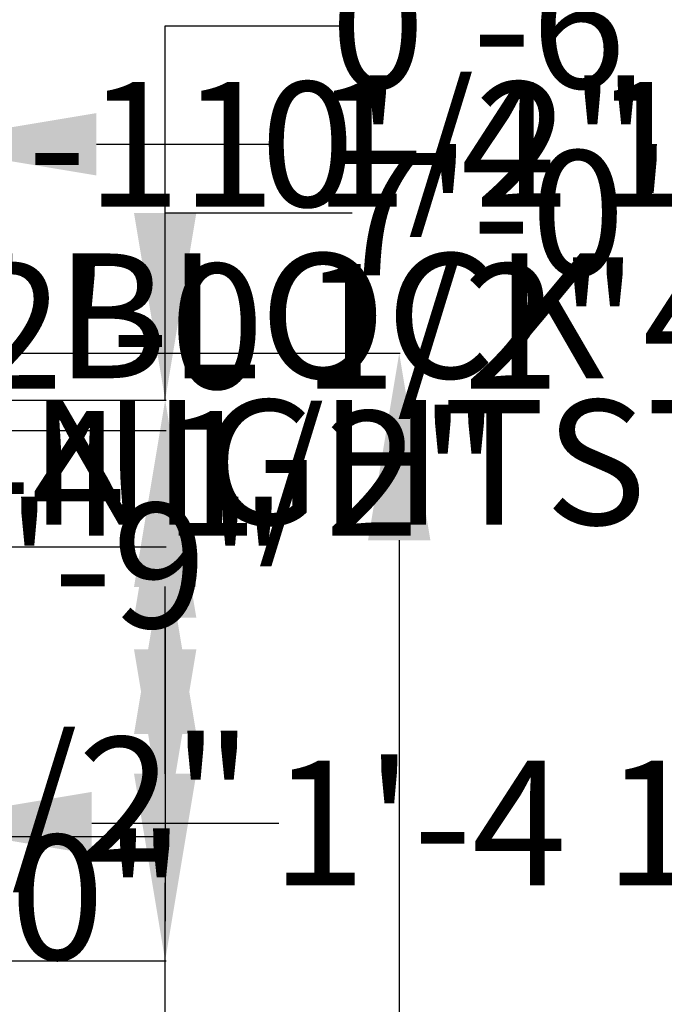
# Model space of a CAD drawing. Units: inches. Extents: x 2838 to 4029, y 1041 to 1915.
# Tile 14 of 16: x 3640 to 3764, y 1546 to 1735. Entities that reach past the tile are written whole.
import ezdxf

# ---------------------------------------------------------------- set-up
doc = ezdxf.new("R2010")
doc.units = ezdxf.units.IN
doc.header["$MEASUREMENT"] = 0
doc.layers.add('A-ANNO-DIMS', color=2, linetype='Continuous', lineweight=18)
doc.styles.get("Standard").update_dxf_attribs({"font": 'arial.ttf'})
doc.dimstyles.get("Standard").update_dxf_attribs({"dimtxt": 24, "dimasz": 36, "dimexe": 0.18, "dimexo": 0.0625, "dimgap": 0.09, "dimtad": 0, "dimtih": 1, "dimtoh": 1, "dimdec": 0, "dimzin": 0, "dimdsep": 46, "dimlunit": 3, "dimtxsty": 'Standard', "dimcen": 0.09, "dimadec": 0, "dimazin": 0, "dimtfac": 1, "dimtdec": 0, "dimtofl": 0, "dimtmove": 0, "dimatfit": 3, "dimfxl": 1, "dimtolj": 1, "dimtzin": 0, "dimarcsym": 0})

# ---------------------------------------------------------------- blocks, each defined once
blk = doc.blocks.new('*D17')
at = {"layer": 'A-ANNO-DIMS', "color": 0, "lineweight": -2, "transparency": 16777216}
for p, q in [((3627.79, 1671.3), (3713.18, 1671.3)), ((3713, 1635.3), (3713, 1443.64)), ((3713, 1227.3), (3713, 1418.95)), ((3627.79, 1191.3), (3713.18, 1191.3))]:
    blk.add_line(p, q, dxfattribs=at)
at = {"layer": 'A-ANNO-DIMS', "color": 0, "transparency": 16777216}
for points in [[(3707, 1635.3), (3719, 1635.3), (3713, 1671.3)], [(3707, 1227.3), (3719, 1227.3), (3713, 1191.3)]]:
    blk.add_solid(points, dxfattribs=at)
at = {"layer": 'Defpoints', "color": 0, "transparency": 16777216}
for p in [(3627.73, 1671.3), (3627.73, 1191.3), (3713, 1191.3)]:
    blk.add_point(p, dxfattribs=at)
at = {"layer": 'A-ANNO-DIMS', "color": 0, "transparency": 16777216, "insert": (3713, 1431.3), "char_height": 24, "attachment_point": 5}
blk.add_mtext("\\A1;40'", dxfattribs=at)
blk = doc.blocks.new('*D27')
at = {"layer": 'A-ANNO-DIMS', "color": 0, "lineweight": -2, "transparency": 16777216}
for p, q in [((3598.68, 1614.31), (3598.68, 1650.31)), ((3598.68, 1650.31), (3634.68, 1650.31)), ((3601.19, 1578.31), (3598.5, 1578.31)), ((3601.19, 1561.16), (3598.5, 1561.16)), ((3598.68, 1525.16), (3598.68, 1489.16))]:
    blk.add_line(p, q, dxfattribs=at)
at = {"layer": 'A-ANNO-DIMS', "color": 0, "transparency": 16777216}
for points in [[(3592.68, 1614.31), (3604.68, 1614.31), (3598.68, 1578.31)], [(3592.68, 1525.16), (3604.68, 1525.16), (3598.68, 1561.16)]]:
    blk.add_solid(points, dxfattribs=at)
at = {"layer": 'Defpoints', "color": 0, "transparency": 16777216}
for p in [(3598.68, 1578.31), (3601.25, 1578.31), (3601.25, 1561.16)]:
    blk.add_point(p, dxfattribs=at)
at = {"layer": 'A-ANNO-DIMS', "color": 0, "transparency": 16777216, "insert": (3820.96, 1650.31), "char_height": 24, "attachment_point": 5}
blk.add_mtext('\\A1;NIGHTSTAND 1\'-5" TYP.', dxfattribs=at)
blk = doc.blocks.new('*D28')
at = {"layer": 'A-ANNO-DIMS', "color": 0, "lineweight": -2, "transparency": 16777216}
for p, q in [((3565.25, 1580.88), (3529.25, 1580.88)), ((3601.25, 1578.37), (3601.25, 1581.06)), ((3617.82, 1578.37), (3617.82, 1581.06)), ((3653.82, 1580.88), (3689.82, 1580.88))]:
    blk.add_line(p, q, dxfattribs=at)
at = {"layer": 'A-ANNO-DIMS', "color": 0, "transparency": 16777216}
for points in [[(3565.25, 1586.88), (3565.25, 1574.88), (3601.25, 1580.88)], [(3653.82, 1586.88), (3653.82, 1574.88), (3617.82, 1580.88)]]:
    blk.add_solid(points, dxfattribs=at)
at = {"layer": 'Defpoints', "color": 0, "transparency": 16777216}
for p in [(3617.82, 1580.88), (3601.25, 1578.31), (3617.82, 1578.31)]:
    blk.add_point(p, dxfattribs=at)
at = {"layer": 'A-ANNO-DIMS', "color": 0, "transparency": 16777216, "insert": (3789.89, 1580.88), "char_height": 24, "attachment_point": 5}
blk.add_mtext('\\A1;1\'-4 1/2" TYP.', dxfattribs=at)
blk = doc.blocks.new('*D36')
at = {"layer": 'A-ANNO-DIMS', "color": 0, "lineweight": -2, "transparency": 16777216}
for p, q in [((3481.95, 1586.87), (3481.95, 1585.25)), ((3488.45, 1586.87), (3488.45, 1585.25)), ((3445.95, 1585.43), (3409.95, 1585.43)), ((3524.45, 1585.43), (3560.45, 1585.43))]:
    blk.add_line(p, q, dxfattribs=at)
at = {"layer": 'A-ANNO-DIMS', "color": 0, "transparency": 16777216}
for points in [[(3445.95, 1591.43), (3445.95, 1579.43), (3481.95, 1585.43)], [(3524.45, 1591.43), (3524.45, 1579.43), (3488.45, 1585.43)]]:
    blk.add_solid(points, dxfattribs=at)
at = {"layer": 'Defpoints', "color": 0, "transparency": 16777216}
for p in [(3481.95, 1586.93), (3488.45, 1586.93), (3488.45, 1585.43)]:
    blk.add_point(p, dxfattribs=at)
at = {"layer": 'A-ANNO-DIMS', "color": 0, "transparency": 16777216, "insert": (3620.4, 1585.43), "char_height": 24, "attachment_point": 5}
blk.add_mtext('\\A1;0\'-6 1/2"', dxfattribs=at)
blk = doc.blocks.new('*D39')
at = {"layer": 'A-ANNO-DIMS', "color": 0, "lineweight": -2, "transparency": 16777216}
for p, q in [((3391.52, 1678.5), (3355.52, 1678.5)), ((3427.52, 1671.36), (3427.52, 1678.68)), ((3475.52, 1671.36), (3475.52, 1678.68)), ((3511.52, 1678.5), (3547.52, 1678.5))]:
    blk.add_line(p, q, dxfattribs=at)
at = {"layer": 'A-ANNO-DIMS', "color": 0, "transparency": 16777216}
for points in [[(3391.52, 1684.5), (3391.52, 1672.5), (3427.52, 1678.5)], [(3511.52, 1684.5), (3511.52, 1672.5), (3475.52, 1678.5)]]:
    blk.add_solid(points, dxfattribs=at)
at = {"layer": 'Defpoints', "color": 0, "transparency": 16777216}
for p in [(3475.52, 1678.5), (3427.52, 1671.3), (3475.52, 1671.3)]:
    blk.add_point(p, dxfattribs=at)
at = {"layer": 'A-ANNO-DIMS', "color": 0, "transparency": 16777216, "insert": (3732.24, 1678.5), "char_height": 24, "attachment_point": 5}
blk.add_mtext('\\A1;VENT BLOCK 4\'-0" TYP.', dxfattribs=at)
blk = doc.blocks.new('*D41')
at = {"layer": 'A-ANNO-DIMS', "color": 0, "lineweight": -2, "transparency": 16777216}
for p, q in [((3284.24, 1506.2), (3284.24, 1496.56)), ((3347.73, 1506.2), (3347.73, 1496.56)), ((3248.24, 1496.74), (3212.24, 1496.74)), ((3383.73, 1496.74), (3419.73, 1496.74))]:
    blk.add_line(p, q, dxfattribs=at)
at = {"layer": 'A-ANNO-DIMS', "color": 0, "transparency": 16777216}
for points in [[(3248.24, 1502.74), (3248.24, 1490.74), (3284.24, 1496.74)], [(3383.73, 1502.74), (3383.73, 1490.74), (3347.73, 1496.74)]]:
    blk.add_solid(points, dxfattribs=at)
at = {"layer": 'Defpoints', "color": 0, "transparency": 16777216}
for p in [(3284.24, 1506.26), (3347.73, 1506.26), (3347.73, 1496.74)]:
    blk.add_point(p, dxfattribs=at)
at = {"layer": 'A-ANNO-DIMS', "color": 0, "transparency": 16777216, "insert": (3624.81, 1496.74), "char_height": 24, "attachment_point": 5}
blk.add_mtext('\\A1;WARDROBE 5\'-3 1/2" TYP.', dxfattribs=at)
blk = doc.blocks.new('*D45')
at = {"layer": 'A-ANNO-DIMS', "color": 0, "lineweight": -2, "transparency": 16777216}
for p, q in [((3456.69, 1635.35), (3456.69, 1630.27)), ((3489.73, 1635.35), (3489.73, 1630.27)), ((3420.69, 1630.45), (3384.69, 1630.45)), ((3525.73, 1630.45), (3561.73, 1630.45))]:
    blk.add_line(p, q, dxfattribs=at)
at = {"layer": 'A-ANNO-DIMS', "color": 0, "transparency": 16777216}
for points in [[(3420.69, 1636.45), (3420.69, 1624.45), (3456.69, 1630.45)], [(3525.73, 1636.45), (3525.73, 1624.45), (3489.73, 1630.45)]]:
    blk.add_solid(points, dxfattribs=at)
at = {"layer": 'Defpoints', "color": 0, "transparency": 16777216}
for p in [(3456.69, 1635.41), (3489.73, 1635.41), (3489.73, 1630.45)]:
    blk.add_point(p, dxfattribs=at)
at = {"layer": 'A-ANNO-DIMS', "color": 0, "transparency": 16777216, "insert": (3626.8, 1630.45), "char_height": 24, "attachment_point": 5}
blk.add_mtext('\\A1;WC 2\'-9"', dxfattribs=at)
blk = doc.blocks.new('*D47')
at = {"layer": 'A-ANNO-DIMS', "color": 0, "lineweight": -2, "transparency": 16777216}
for p, q in [((3493.47, 1640.5), (3493.47, 1676.5)), ((3493.47, 1676.5), (3529.47, 1676.5)), ((3489.85, 1604.5), (3493.65, 1604.5)), ((3489.85, 1579.95), (3493.65, 1579.95)), ((3493.47, 1543.95), (3493.47, 1507.95))]:
    blk.add_line(p, q, dxfattribs=at)
at = {"layer": 'A-ANNO-DIMS', "color": 0, "transparency": 16777216}
for points in [[(3487.47, 1640.5), (3499.47, 1640.5), (3493.47, 1604.5)], [(3487.47, 1543.95), (3499.47, 1543.95), (3493.47, 1579.95)]]:
    blk.add_solid(points, dxfattribs=at)
at = {"layer": 'Defpoints', "color": 0, "transparency": 16777216}
for p in [(3489.78, 1604.5), (3493.47, 1604.5), (3489.78, 1579.95)]:
    blk.add_point(p, dxfattribs=at)
at = {"layer": 'A-ANNO-DIMS', "color": 0, "transparency": 16777216, "insert": (3643.85, 1676.5), "char_height": 24, "attachment_point": 5}
blk.add_mtext('\\A1;BASIN 2\'-0 1/2"', dxfattribs=at)
blk = doc.blocks.new('*D56')
at = {"layer": 'A-ANNO-DIMS', "color": 0, "lineweight": -2, "transparency": 16777216}
for p, q in [((3567.44, 1530.6), (3567.44, 1566.6)), ((3567.44, 1566.6), (3603.44, 1566.6)), ((3562.33, 1494.6), (3567.62, 1494.6)), ((3562.33, 1470.6), (3567.62, 1470.6)), ((3567.44, 1434.6), (3567.44, 1398.6))]:
    blk.add_line(p, q, dxfattribs=at)
at = {"layer": 'A-ANNO-DIMS', "color": 0, "transparency": 16777216}
for points in [[(3561.44, 1530.6), (3573.44, 1530.6), (3567.44, 1494.6)], [(3561.44, 1434.6), (3573.44, 1434.6), (3567.44, 1470.6)]]:
    blk.add_solid(points, dxfattribs=at)
at = {"layer": 'Defpoints', "color": 0, "transparency": 16777216}
for p in [(3562.26, 1494.6), (3567.44, 1494.6), (3562.26, 1470.6)]:
    blk.add_point(p, dxfattribs=at)
at = {"layer": 'A-ANNO-DIMS', "color": 0, "transparency": 16777216, "insert": (3635.63, 1566.6), "char_height": 24, "attachment_point": 5}
blk.add_mtext('\\A1;2\'-0"', dxfattribs=at)
blk = doc.blocks.new('*D73')
at = {"layer": 'A-ANNO-DIMS', "color": 0, "lineweight": -2, "transparency": 16777216}
for p, q in [((3425.038746, 1711.522346), (3389.038746, 1711.522346)), ((3461.038746, 1200.359846), (3461.038746, 1711.702346)), ((3618.731626, 1200.359846), (3618.731626, 1711.702346)), ((3654.731626, 1711.522346), (3690.731626, 1711.522346))]:
    blk.add_line(p, q, dxfattribs=at)
at = {"layer": 'A-ANNO-DIMS', "color": 0, "transparency": 16777216}
for points in [[(3425.038746, 1717.522346), (3425.038746, 1705.522346), (3461.038746, 1711.522346)], [(3654.731626, 1717.522346), (3654.731626, 1705.522346), (3618.731626, 1711.522346)]]:
    blk.add_solid(points, dxfattribs=at)
at = {"layer": 'Defpoints', "color": 0, "transparency": 16777216}
for p in [(3618.731626, 1711.522346), (3461.038746, 1200.297346), (3618.731626, 1200.297346)]:
    blk.add_point(p, dxfattribs=at)
at = {"layer": 'A-ANNO-DIMS', "color": 0, "transparency": 16777216, "insert": (3539.885186, 1711.522346), "char_height": 24, "attachment_point": 5}
blk.add_mtext('\\A1;13\'-1 1/2"', dxfattribs=at)
blk = doc.blocks.new('*D78')
at = {"layer": 'A-ANNO-DIMS', "color": 0, "lineweight": -2, "transparency": 16777216}
for p, q in [((3667.956626, 1590.394218), (3667.956626, 1626.394218)), ((3498.794126, 1554.394218), (3668.136626, 1554.394218)), ((3498.638013, 1506.394218), (3668.136626, 1506.394218)), ((3667.956626, 1470.394218), (3667.956626, 1434.394218))]:
    blk.add_line(p, q, dxfattribs=at)
at = {"layer": 'A-ANNO-DIMS', "color": 0, "transparency": 16777216}
for points in [[(3661.956626, 1590.394218), (3673.956626, 1590.394218), (3667.956626, 1554.394218)], [(3661.956626, 1470.394218), (3673.956626, 1470.394218), (3667.956626, 1506.394218)]]:
    blk.add_solid(points, dxfattribs=at)
at = {"layer": 'Defpoints', "color": 0, "transparency": 16777216}
for p in [(3498.731626, 1554.394218), (3667.956626, 1554.394218), (3498.575513, 1506.394218)]:
    blk.add_point(p, dxfattribs=at)
at = {"layer": 'A-ANNO-DIMS', "color": 0, "transparency": 16777216, "insert": (3667.956626, 1530.394218), "char_height": 24, "attachment_point": 5}
blk.add_mtext('\\A1;4\'-0"', dxfattribs=at)
blk = doc.blocks.new('*D84')
at = {"layer": 'A-ANNO-DIMS', "color": 0, "lineweight": -2, "transparency": 16777216}
for p, q in [((3667.96, 1662.3), (3667.96, 1698.3)), ((3667.96, 1698.3), (3703.96, 1698.3)), ((3489.79, 1662.3), (3668.14, 1662.3)), ((3667.96, 1614.3), (3667.96, 1626.3)), ((3489.79, 1578.3), (3668.14, 1578.3))]:
    blk.add_line(p, q, dxfattribs=at)
at = {"layer": 'A-ANNO-DIMS', "color": 0, "transparency": 16777216}
for points in [[(3661.96, 1626.3), (3673.96, 1626.3), (3667.96, 1662.3)], [(3661.96, 1614.3), (3673.96, 1614.3), (3667.96, 1578.3)]]:
    blk.add_solid(points, dxfattribs=at)
at = {"layer": 'Defpoints', "color": 0, "transparency": 16777216}
for p in [(3489.73, 1662.3), (3667.96, 1662.3), (3489.73, 1578.3)]:
    blk.add_point(p, dxfattribs=at)
at = {"layer": 'A-ANNO-DIMS', "color": 0, "transparency": 16777216, "insert": (3735.85, 1698.3), "char_height": 24, "attachment_point": 5}
blk.add_mtext('\\A1;7\'-0"', dxfattribs=at)
blk = doc.blocks.new('*D94')
at = {"layer": 'A-ANNO-DIMS', "color": 0, "lineweight": -2, "transparency": 16777216}
for p, q in [((3667.96, 1533.39), (3667.96, 1569.39)), ((3585.44, 1497.39), (3668.14, 1497.39)), ((3585.44, 1469.25), (3668.14, 1469.25)), ((3667.96, 1433.25), (3667.96, 1397.25))]:
    blk.add_line(p, q, dxfattribs=at)
at = {"layer": 'A-ANNO-DIMS', "color": 0, "transparency": 16777216}
for points in [[(3661.96, 1533.39), (3673.96, 1533.39), (3667.96, 1497.39)], [(3661.96, 1433.25), (3673.96, 1433.25), (3667.96, 1469.25)]]:
    blk.add_solid(points, dxfattribs=at)
at = {"layer": 'Defpoints', "color": 0, "transparency": 16777216}
for p in [(3585.37, 1497.39), (3585.37, 1469.25), (3667.96, 1469.25)]:
    blk.add_point(p, dxfattribs=at)
at = {"layer": 'A-ANNO-DIMS', "color": 0, "transparency": 16777216, "insert": (3667.96, 1483.32), "char_height": 24, "attachment_point": 5}
blk.add_mtext('\\A1;2\'-4"', dxfattribs=at)
blk = doc.blocks.new('*D96')
at = {"layer": 'A-ANNO-DIMS', "color": 0, "lineweight": -2, "transparency": 16777216}
for p, q in [((3462.73, 1711.52), (3426.73, 1711.52)), ((3498.73, 1662.36), (3498.73, 1711.7)), ((3546.42, 1662.36), (3546.42, 1711.7)), ((3582.42, 1711.52), (3618.42, 1711.52))]:
    blk.add_line(p, q, dxfattribs=at)
at = {"layer": 'A-ANNO-DIMS', "color": 0, "transparency": 16777216}
for points in [[(3462.73, 1717.52), (3462.73, 1705.52), (3498.73, 1711.52)], [(3582.42, 1717.52), (3582.42, 1705.52), (3546.42, 1711.52)]]:
    blk.add_solid(points, dxfattribs=at)
at = {"layer": 'Defpoints', "color": 0, "transparency": 16777216}
for p in [(3546.42, 1711.52), (3498.73, 1662.3), (3546.42, 1662.3)]:
    blk.add_point(p, dxfattribs=at)
at = {"layer": 'A-ANNO-DIMS', "color": 0, "transparency": 16777216, "insert": (3687.68, 1711.52), "char_height": 24, "attachment_point": 5}
blk.add_mtext('\\A1;3\'-11 1/2"', dxfattribs=at)
blk = doc.blocks.new('*D97')
at = {"layer": 'A-ANNO-DIMS', "color": 0, "lineweight": -2, "transparency": 16777216}
for p, q in [((3667.956626, 1698.297346), (3667.956626, 1734.297346)), ((3618.794126, 1662.297346), (3668.136626, 1662.297346)), ((3618.794126, 1634.032994), (3668.136626, 1634.032994)), ((3667.956626, 1598.032994), (3667.956626, 1562.032994))]:
    blk.add_line(p, q, dxfattribs=at)
at = {"layer": 'A-ANNO-DIMS', "color": 0, "transparency": 16777216}
for points in [[(3661.956626, 1698.297346), (3673.956626, 1698.297346), (3667.956626, 1662.297346)], [(3661.956626, 1598.032994), (3673.956626, 1598.032994), (3667.956626, 1634.032994)]]:
    blk.add_solid(points, dxfattribs=at)
at = {"layer": 'Defpoints', "color": 0, "transparency": 16777216}
for p in [(3618.731626, 1662.297346), (3618.731626, 1634.032994), (3667.956626, 1634.032994)]:
    blk.add_point(p, dxfattribs=at)
at = {"layer": 'A-ANNO-DIMS', "color": 0, "transparency": 16777216, "insert": (3667.956626, 1648.16517), "char_height": 24, "attachment_point": 5}
blk.add_mtext('\\A1;2\'-4 1/2"', dxfattribs=at)
blk = doc.blocks.new('*D102')
at = {"layer": 'A-ANNO-DIMS', "color": 0, "lineweight": -2, "transparency": 16777216}
for p, q in [((3667.96, 1698.3), (3667.96, 1734.3)), ((3667.96, 1734.3), (3703.96, 1734.3)), ((3489.79, 1662.3), (3668.14, 1662.3)), ((3489.79, 1656.41), (3668.14, 1656.41)), ((3667.96, 1620.41), (3667.96, 1584.41))]:
    blk.add_line(p, q, dxfattribs=at)
at = {"layer": 'A-ANNO-DIMS', "color": 0, "transparency": 16777216}
for points in [[(3661.96, 1698.3), (3673.96, 1698.3), (3667.96, 1662.3)], [(3661.96, 1620.41), (3673.96, 1620.41), (3667.96, 1656.41)]]:
    blk.add_solid(points, dxfattribs=at)
at = {"layer": 'Defpoints', "color": 0, "transparency": 16777216}
for p in [(3489.73, 1662.3), (3667.96, 1662.3), (3489.73, 1656.41)]:
    blk.add_point(p, dxfattribs=at)
at = {"layer": 'A-ANNO-DIMS', "color": 0, "transparency": 16777216, "insert": (3735.95, 1734.3), "char_height": 24, "attachment_point": 5}
blk.add_mtext('\\A1;0\'-6"', dxfattribs=at)
blk = doc.blocks.new('*D104')
at = {"layer": 'A-ANNO-DIMS', "color": 0, "lineweight": -2, "transparency": 16777216}
for p, q in [((3667.956626, 1533.394218), (3667.956626, 1569.394218)), ((3618.794126, 1497.394218), (3668.136626, 1497.394218)), ((3614.522024, 1472.357294), (3668.136626, 1472.357294)), ((3667.956626, 1436.357294), (3667.956626, 1400.357294))]:
    blk.add_line(p, q, dxfattribs=at)
at = {"layer": 'A-ANNO-DIMS', "color": 0, "transparency": 16777216}
for points in [[(3661.956626, 1533.394218), (3673.956626, 1533.394218), (3667.956626, 1497.394218)], [(3661.956626, 1436.357294), (3673.956626, 1436.357294), (3667.956626, 1472.357294)]]:
    blk.add_solid(points, dxfattribs=at)
at = {"layer": 'Defpoints', "color": 0, "transparency": 16777216}
for p in [(3618.731626, 1497.394218), (3614.459524, 1472.357294), (3667.956626, 1472.357294)]:
    blk.add_point(p, dxfattribs=at)
at = {"layer": 'A-ANNO-DIMS', "color": 0, "transparency": 16777216, "insert": (3667.956626, 1484.875756), "char_height": 24, "attachment_point": 5}
blk.add_mtext('\\A1;2\'-1"', dxfattribs=at)
blk = doc.blocks.new('*D105')
at = {"layer": 'A-ANNO-DIMS', "color": 0, "lineweight": -2, "transparency": 16777216}
for p, q in [((3578.46, 1711.52), (3542.46, 1711.52)), ((3614.46, 1472.42), (3614.46, 1711.7)), ((3618.73, 1469.91), (3618.73, 1711.7)), ((3654.73, 1711.52), (3690.73, 1711.52))]:
    blk.add_line(p, q, dxfattribs=at)
at = {"layer": 'A-ANNO-DIMS', "color": 0, "transparency": 16777216}
for points in [[(3578.46, 1717.52), (3578.46, 1705.52), (3614.46, 1711.52)], [(3654.73, 1717.52), (3654.73, 1705.52), (3618.73, 1711.52)]]:
    blk.add_solid(points, dxfattribs=at)
at = {"layer": 'Defpoints', "color": 0, "transparency": 16777216}
for p in [(3618.73, 1711.52), (3614.46, 1472.36), (3618.73, 1469.85)]:
    blk.add_point(p, dxfattribs=at)
at = {"layer": 'A-ANNO-DIMS', "color": 0, "transparency": 16777216, "insert": (3750.68, 1711.52), "char_height": 24, "attachment_point": 5}
blk.add_mtext('\\A1;0\'-4 1/2"', dxfattribs=at)

msp = doc.modelspace()

# ---------------------------------------------------------------- dimensions: what is measured, and where the dimension line sits
at = {"layer": 'A-ANNO-DIMS'}
for base, p1, p2, text, picture, middle in [((3475.52, 1678.5), (3427.52, 1671.3), (3475.52, 1671.3), 'VENT BLOCK <> TYP.', '*D39', (3732.24, 1678.5)), ((3489.73, 1630.45), (3456.69, 1635.41), (3489.73, 1635.41), 'WC <>', '*D45', (3626.8, 1630.45)), ((3617.82, 1580.88), (3601.25, 1578.31), (3617.82, 1578.31), '<> TYP.', '*D28', (3789.89, 1580.88)), ((3347.73, 1496.74), (3284.24, 1506.26), (3347.73, 1506.26), 'WARDROBE <> TYP.', '*D41', (3624.81, 1496.74))]:
    dim = msp.add_linear_dim(base=base, p1=p1, p2=p2, text=text, dimstyle='Standard', override={"dimdec": 1, "dimlfac": 1, "dimrnd": 0, "dimzin": 1, "dimdsep": 46, "dimlunit": 4, "dimfrac": 2}, dxfattribs=at)
    dim.commit()
    dim.dimension.update_dxf_attribs({"geometry": picture, "text_midpoint": middle})
for base, p1, p2, override, picture, middle in [((3667.96, 1662.3), (3489.73, 1656.41), (3489.73, 1662.3), {"dimdec": 1, "dimlfac": 1, "dimrnd": 0, "dimzin": 1, "dimdsep": 46, "dimlunit": 4, "dimfrac": 2}, '*D102', (3735.95, 1734.3)), ((3667.96, 1634.03), (3618.73, 1662.3), (3618.73, 1634.03), {"dimdec": 1, "dimlfac": 1, "dimrnd": 0, "dimzin": 1, "dimdsep": 46, "dimlunit": 4, "dimfrac": 2}, '*D97', (3667.96, 1648.17)), ((3667.96, 1662.3), (3489.73, 1578.3), (3489.73, 1662.3), {"dimdec": 1, "dimlfac": 1, "dimrnd": 0, "dimzin": 1, "dimdsep": 46, "dimlunit": 4, "dimfrac": 2}, '*D84', (3735.85, 1698.3)), ((3713, 1191.3), (3627.73, 1671.3), (3627.73, 1191.3), {"dimclrd": 0, "dimclre": 0, "dimclrt": 0}, '*D17', (3713, 1431.3)), ((3667.96, 1554.39), (3498.58, 1506.39), (3498.73, 1554.39), {"dimdec": 1, "dimlfac": 1, "dimrnd": 0, "dimzin": 1, "dimdsep": 46, "dimlunit": 4, "dimfrac": 2}, '*D78', (3667.96, 1530.39)), ((3567.44, 1494.6), (3562.26, 1470.6), (3562.26, 1494.6), {"dimdec": 1, "dimlfac": 1, "dimrnd": 0, "dimzin": 1, "dimdsep": 46, "dimlunit": 4, "dimfrac": 2}, '*D56', (3635.63, 1566.6)), ((3667.96, 1469.25), (3585.37, 1497.39), (3585.37, 1469.25), {"dimdec": 1, "dimlfac": 1, "dimrnd": 0, "dimzin": 1, "dimdsep": 46, "dimlunit": 4, "dimfrac": 2}, '*D94', (3667.96, 1483.32)), ((3667.96, 1472.36), (3618.73, 1497.39), (3614.46, 1472.36), {"dimdec": 1, "dimlfac": 1, "dimrnd": 0, "dimzin": 1, "dimdsep": 46, "dimlunit": 4, "dimfrac": 2}, '*D104', (3667.96, 1484.88))]:
    dim = msp.add_linear_dim(base=base, p1=p1, p2=p2, angle=90, dimstyle='Standard', override=override, dxfattribs=at)
    dim.commit()
    dim.dimension.update_dxf_attribs({"geometry": picture, "text_midpoint": middle})
for base, p1, p2, picture, middle in [((3618.73, 1711.52), (3461.04, 1200.3), (3618.73, 1200.3), '*D73', (3539.89, 1711.52)), ((3546.42, 1711.52), (3498.73, 1662.3), (3546.42, 1662.3), '*D96', (3687.68, 1711.52)), ((3618.73, 1711.52), (3614.46, 1472.36), (3618.73, 1469.85), '*D105', (3750.68, 1711.52)), ((3488.45, 1585.43), (3481.95, 1586.93), (3488.45, 1586.93), '*D36', (3620.4, 1585.43))]:
    dim = msp.add_linear_dim(base=base, p1=p1, p2=p2, dimstyle='Standard', override={"dimdec": 1, "dimlfac": 1, "dimrnd": 0, "dimzin": 1, "dimdsep": 46, "dimlunit": 4, "dimfrac": 2}, dxfattribs=at)
    dim.commit()
    dim.dimension.update_dxf_attribs({"geometry": picture, "text_midpoint": middle})
for base, p1, p2, text, picture, middle in [((3493.4667, 1604.5013), (3489.7841, 1579.9504), (3489.7841, 1604.5013), 'BASIN <>', '*D47', (3643.8514, 1676.5013)), ((3598.6826, 1578.3092), (3601.2549, 1561.1604), (3601.2549, 1578.3092), 'NIGHTSTAND <> TYP.', '*D27', (3820.9609, 1650.3092))]:
    dim = msp.add_linear_dim(base=base, p1=p1, p2=p2, angle=90, text=text, dimstyle='Standard', override={"dimdec": 1, "dimlfac": 1, "dimrnd": 0, "dimzin": 1, "dimdsep": 46, "dimlunit": 4, "dimfrac": 2}, dxfattribs=at)
    dim.commit()
    dim.dimension.update_dxf_attribs({"geometry": picture, "text_midpoint": middle})

doc.saveas('drawing.dxf')
